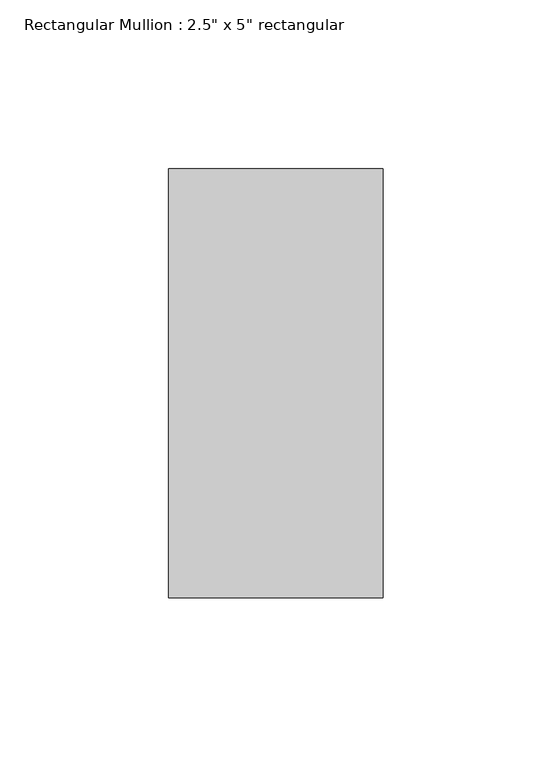
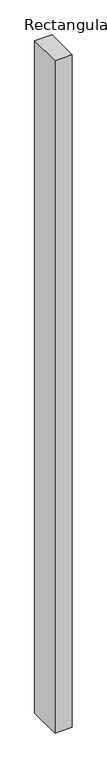
"""IFC4 building model written with IfcOpenShell, lengths in millimetres: member geometry."""

from ifc_helpers import new_model, si_unit, frame, origin, place, context, project, spatial, polyline, outline, extrude, source, transform, mapped, element, save


def member_9f3fc137(model_context):
    return source(origin(), model_context, "Body", "SweptSolid", [
        extrude(outline(polyline([(0.0, 63.5), (0.0, -63.5), (-63.5, -63.5), (-63.5, 63.5), (0.0, 63.5)])), frame((0.0, 0.0, -2590.8), z_axis=(0.0, 0.0, 1.0), x_axis=(1.0, 0.0, 0.0)), (0.0, 0.0, 1.0), 2590.8),
    ])


if __name__ == "__main__":
    model = new_model("IFC4")
    model_context = context("Model", 3, world=origin())
    ifc_project = project(units=[si_unit("LENGTHUNIT", "METRE", prefix="MILLI")], contexts=[model_context])
    site = spatial("IfcSite", under=ifc_project)
    building = spatial("IfcBuilding", under=site)
    placement = place(None, origin())
    member_shape = member_9f3fc137(model_context)
    element("IfcMember", 1, ObjectType="Rectangular Mullion : 2.5\" x 5\" rectangular", at=placement, inside=building, context=model_context, shape_type="MappedRepresentation", body=[
        mapped(member_shape, transform((0.0, 0.0, 0.0), x_axis=(1.0, 0.0, 0.0), y_axis=(0.0, 1.0, 0.0), z_axis=(0.0, 0.0, 1.0))),
    ])
    save(model, "model.ifc")

# Revit data of these elements
# Type "Rectangular Mullion : 2.5\" x 5\" rectangular"
#   built-in parameter 1007304 = 0.416667 (stored number, unit not read)
#   built-in parameter 1007301 = 0.104167 (stored number, unit not read)
#   built-in parameter 1007300 = 0.104167 (stored number, unit not read)
# Element 1 (IfcMember, "Rectangular Mullion : 2.5\" x 5\" rectangular")
#   Materials on its faces: "Aluminum"
# Materials
#   "Aluminum": class "Metal", colour RGB 247 247 247, transparency 0, Description = "Aluminum 6061", Cost = 0
